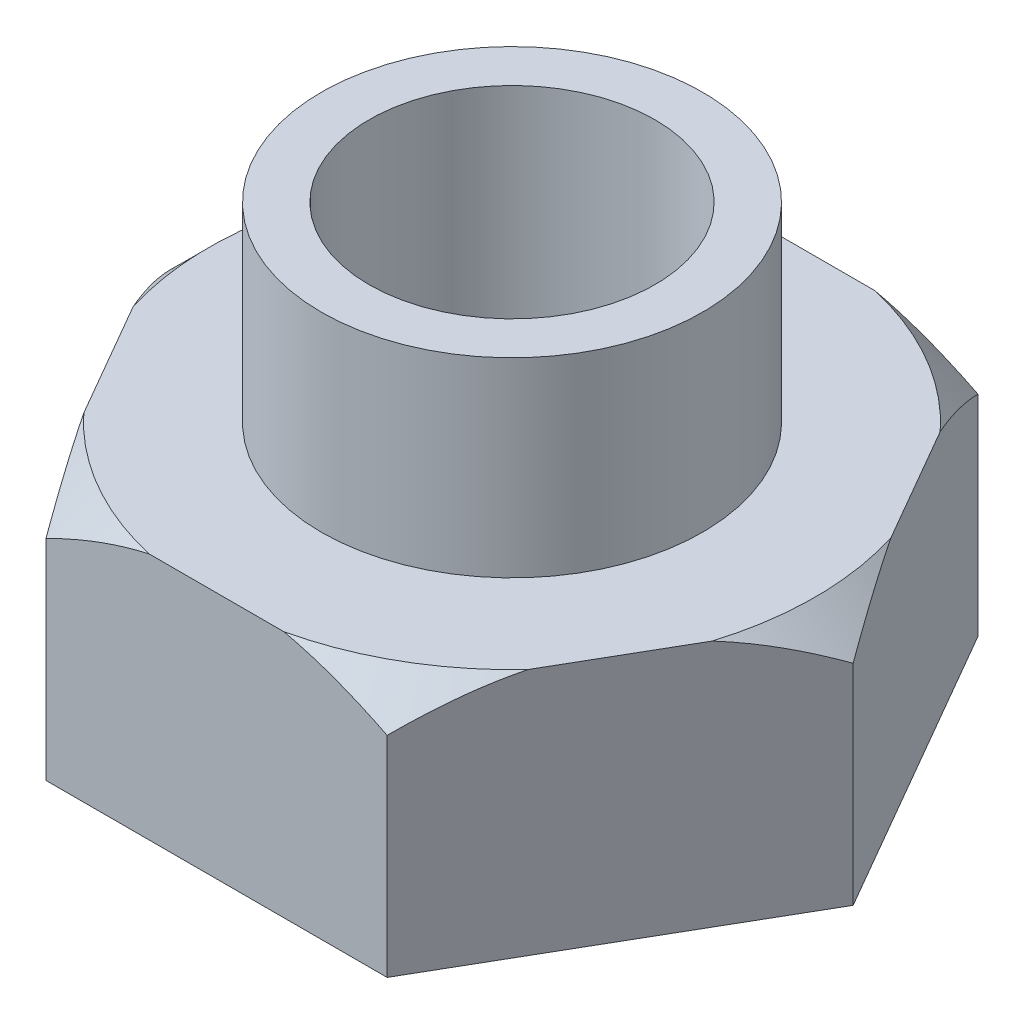
from build123d import *

# Parameters (mm, degrees)
HEX_BODY_155AF_X65_DEPTH = 65
COLLAR_PROFILE_100_R     = 50
COLLAR_100_X50_DEPTH     = 50
THROUGH_BORE_75_REACH    = 167.044
BORE_PROFILE_75_R        = 37.5


with BuildPart() as part:
    # Hex Profile 155AF → Hex Body 155AF x65 (new body)
    with BuildSketch(Plane(origin=(0, 0, 0), x_dir=(1, 0, 0), z_dir=(0, 1, 0))):
        Polygon((89.489291724, 0), (44.744645862, 77.5), (-44.744645862, 77.5), (-89.489291724, 0), (-44.744645862, -77.5), (44.744645862, -77.5), align=None)
    extrude(amount=HEX_BODY_155AF_X65_DEPTH)

    # Hex Chamfer Profile 10x10 → Hex Corner Chamfer 10x10 (revolve, cut)
    with BuildSketch(Plane.XY):
        Polygon((79.489291724, 65), (89.489291724, 65), (89.489291724, 55), align=None)
    revolve(axis=Axis((0, 0, 0), (0, 1, 0)), mode=Mode.SUBTRACT)

    # Collar Profile Ø100 → Collar Ø100 x50 (add)
    with BuildSketch(Plane(origin=(0, 65, 0), x_dir=(1, 0, 0), z_dir=(0, 1, 0))):
        with Locations(Location((0, 0, 0), (0, 0, 270))):
            Circle(COLLAR_PROFILE_100_R)
    extrude(amount=COLLAR_100_X50_DEPTH)

    # Bore Profile Ø75 → Through Bore Ø75 (cut, up to next)
    with BuildSketch(Plane(origin=(0, 115, 0), x_dir=(1, 0, 0), z_dir=(0, 1, 0)), mode=Mode.PRIVATE) as through_bore_75_sk1:
        with Locations(Location((0, 0, 0), (0, 0, 270))):
            Circle(BORE_PROFILE_75_R)
    through_bore_75_tool1 = extrude(through_bore_75_sk1.sketch, amount=-THROUGH_BORE_75_REACH, mode=Mode.PRIVATE) & part.part
    add(through_bore_75_tool1.solids().sort_by_distance((0, 115, 0))[0], mode=Mode.SUBTRACT)


solid = part.part
